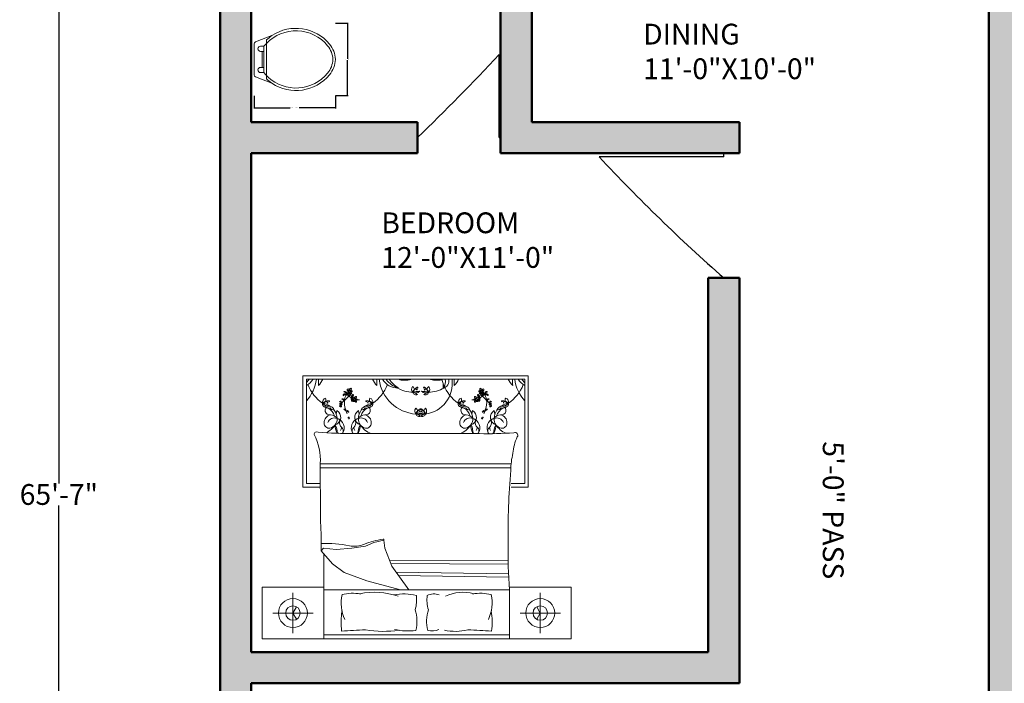
# Model space of a CAD drawing. Units: inches. Extents: x -17 to 536, y -817 to 53.
# Tile 4 of 9: x -17 to 268, y -436 to -245. Entities that reach past the tile are written whole.
import ezdxf

# ---------------------------------------------------------------- set-up
doc = ezdxf.new("R2010")
doc.units = ezdxf.units.IN
doc.header["$MEASUREMENT"] = 0
for name, color, linetype, lineweight in [('A-ANNO-DIMS', 2, 'Continuous', 18), ('A-AREA-IDEN', 7, 'Continuous', 18), ('A-DOOR', 4, 'Continuous', 25), ('A-FLOR-FIXT', 9, 'Continuous', 18), ('A-FURN', 8, 'Continuous', 13), ('A-WALL', 7, 'Continuous', 50), ('A-WALL-PATT', 22, 'Continuous', 13)]:
    doc.layers.add(name, color=color, linetype=linetype, lineweight=lineweight)
doc.styles.get("Standard").update_dxf_attribs({"font": 'arial.ttf'})
doc.dimstyles.get("Standard").update_dxf_attribs({"dimtxt": 0.18, "dimasz": 0.18, "dimexe": 0.18, "dimexo": 0.0625, "dimgap": 0.09, "dimtad": 0, "dimtih": 1, "dimtoh": 1, "dimdec": 0, "dimzin": 0, "dimdsep": 46, "dimlunit": 3, "dimtxsty": 'Standard', "dimcen": 0.09, "dimadec": 0, "dimazin": 0, "dimtfac": 1, "dimtdec": 0, "dimtofl": 0, "dimtmove": 0, "dimatfit": 3, "dimfxl": 1, "dimtolj": 1, "dimtzin": 0, "dimarcsym": 0})

# ---------------------------------------------------------------- blocks, each defined once
blk = doc.blocks.new('*D2')
at = {"layer": 'A-ANNO-DIMS', "color": 0, "lineweight": -2, "transparency": 16777216}
for p, q in [((41.3, 11.55), (-5.38, 11.55)), ((-5.2, 11.37), (-5.2, -378.8)), ((-5.2, -775.27), (-5.2, -385.1)), ((41.3, -775.45), (-5.38, -775.45))]:
    blk.add_line(p, q, dxfattribs=at)
at = {"layer": 'A-ANNO-DIMS', "color": 0, "transparency": 16777216}
for points in [[(-5.23, 11.37), (-5.17, 11.37), (-5.2, 11.55)], [(-5.23, -775.27), (-5.17, -775.27), (-5.2, -775.45)]]:
    blk.add_solid(points, dxfattribs=at)
at = {"layer": 'Defpoints', "color": 0, "transparency": 16777216}
for p in [(41.37, 11.55), (-5.2, -775.45), (41.37, -775.45)]:
    blk.add_point(p, dxfattribs=at)
at = {"layer": 'A-ANNO-DIMS', "color": 0, "transparency": 16777216, "insert": (-5.2, -381.95), "char_height": 6, "attachment_point": 5}
blk.add_mtext('\\A1;65\'-7"', dxfattribs=at)
blk = doc.blocks.new('BED-WITH-NIGHTSTANDS-STANDARD')
for p, q in [((11.79, 75.95), (11.79, 43.78)), ((76.89, 75.95), (11.79, 75.95)), ((12.82, 74.91), (75.86, 74.91)), ((12.82, 44.81), (12.82, 74.91)), ((75.86, 74.91), (75.86, 44.81)), ((76.89, 43.78), (76.89, 75.95)), ((21.62, 65.86), (21.42, 64.85)), ((27.86, 65.86), (28.06, 64.85)), ((60.82, 65.86), (60.62, 64.85)), ((67.06, 65.86), (67.25, 64.85)), ((62.78, 59.23), (26.52, 59.23)), ((71.93, 50.46), (16.83, 50.46)), ((71.85, 49.35), (16.83, 49.35)), ((11.79, 43.78), (16.84, 43.78)), ((16.84, 44.81), (12.82, 44.81)), ((75.86, 44.81), (71.92, 44.81)), ((71.94, 43.78), (76.89, 43.78)), ((35.15, 28.52), (32.25, 27.79)), ((35.51, 26.17), (35.15, 28.52)), ((17.78, 26.17), (17.06, 25.44)), ((21.4, 25.8), (17.78, 26.17)), ((25.92, 26.17), (21.4, 25.8)), ((29.9, 26.71), (25.92, 26.17)), ((32.25, 27.79), (29.9, 26.71)), ((37.5, 20.92), (35.51, 26.17)), ((17.06, 25.44), (20.32, 21.65)), ((17.86, 0), (17.86, 24.51)), ((20.32, 21.65), (23.75, 19.12)), ((71.13, 22.47), (36.86, 22.61)), ((71.12, 21.55), (37.21, 21.69)), ((42.39, 14.11), (37.5, 20.92)), ((23.75, 19.12), (30.26, 16.77)), ((71.17, 18.74), (38.74, 19.2)), ((71.2, 17.82), (39.41, 18.27)), ((30.26, 16.77), (40, 14.11)), ((8.93, 13.28), (8.93, 1.61)), ((17.86, 14.11), (71.44, 14.11)), ((80.37, 13.28), (80.37, 1.61)), ((14.76, 7.44), (3.1, 7.44)), ((74.54, 7.44), (86.21, 7.44)), ((0, 0), (89.3, 0)), ((71.44, 1.15), (17.86, 1.15))]:
    blk.add_line(p, q)
for points in [[(16.87, 33.62, -0.001242), (16.83, 50.56, 0.127202), (15.04, 59.01)], [(71.82, 48.64, -0.056112), (72.47, 53.56, -0.095341), (73.73, 58.29)], [(22.99, 2.23, -0.074897), (23.1, 8.06, 0.472817)], [(44.23, 8.39, -0.14099), (44.41, 2.43, -0.235245)], [(48.05, 8.39, 0.14099), (47.87, 2.43, 0.235245)], [(66.31, 2.23, 0.074897), (66.2, 8.06, -0.472817)]]:
    blk.add_lwpolyline(points, format="xyb")
for points in [[(17.86, 14.88), (0, 14.88), (0, 0)], [(71.44, 0), (71.44, 14.88), (89.3, 14.88), (89.3, 0)], [(8.93, 7.44), (9.97, 9.25)], [(80.37, 7.44), (79.33, 9.25)], [(8.93, 7.44), (9.97, 5.64)], [(80.37, 7.44), (79.33, 5.64)]]:
    blk.add_lwpolyline(points)
for centre, radius in [((25.29, 71.49), 0.227), ((63.39, 71.49), 0.227), ((26.78, 69.09), 0.227), ((61.9, 69.09), 0.227), ((8.93, 7.44), 4.17), ((80.37, 7.44), 4.17), ((8.93, 7.44), 2.08), ((80.37, 7.44), 2.08)]:
    blk.add_circle(centre, radius)
for centre, radius, start, end in [((7.95, 79.1), 7.08, 313.5186, 323.6964), ((9.99, 78.04), 5.68, 299.8884, 326.5383), ((4.14, 76.48), 11.66, 318.1144, 352.255), ((13.17, 76.73), 4.74, 311.0454, 337.4453), ((0.19, 74.18), 16.13, 356.3481, 2.5919), ((36.31, 76.73), 4.74, 202.5547, 228.9546), ((49.3, 74.18), 16.13, 177.4081, 183.6519), ((45.35, 76.48), 11.66, 187.745, 265.5377), ((39.5, 78.04), 5.68, 213.4617, 268.728), ((41.54, 79.1), 7.08, 216.3036, 252.1496), ((45.26, 81.09), 10.53, 215.947, 235.9877), ((41.19, 81.04), 6.41, 252.9798, 286.4569), ((43.73, 84.35), 9.48, 264.3643, 265.6213), ((48.73, 90.84), 16.94, 250.0972, 250.2783), ((45.93, 73.79), 9.03, 278.1803, 7.1364), ((50.46, 81.04), 6.41, 253.5431, 287.0202), ((47.92, 84.35), 9.48, 274.3787, 275.6357), ((42.93, 90.84), 16.94, 289.7217, 289.9028), ((47.1, 72.96), 5.22, 353.3805, 21.883), ((51.89, 74.42), 2.09, 280.9261, 13.6102), ((50.32, 74.13), 2.65, 318.0951, 17.1391), ((39.38, 74.18), 16.13, 356.3481, 2.5919), ((52.37, 76.73), 4.74, 311.0454, 337.4453), ((75.51, 76.73), 4.74, 202.5547, 228.9546), ((88.49, 74.18), 16.13, 177.4081, 183.6519), ((84.54, 76.48), 11.66, 187.745, 221.8856), ((78.69, 78.04), 5.68, 213.4617, 240.1116), ((80.73, 79.1), 7.08, 216.3036, 226.4814), ((24.09, 77.63), 11.66, 201.4092, 235.6135), ((23.83, 71.16), 0.254, 55.6077, 145.6462), ((23.65, 70.61), 0.687, 21.7087, 93.0299), ((20.03, 65.71), 6.64, 53.6254, 57.3216), ((23.86, 70.79), 0.592, 342.8042, 79.6943), ((24.82, 71.92), 0.225, 134.3732, 211.9501), ((25.23, 72.18), 0.717, 211.9501, 255.2442), ((24.83, 71.66), 0.449, 8.5614, 112.5914), ((25.04, 71.17), 0.31, 88.5719, 233.8954), ((25.01, 71.09), 0.223, 228.2946, 6.2474), ((24.96, 71.68), 0.151, 352.868, 97.094), ((24.8, 71.35), 0.313, 298.8493, 359.9355), ((24.87, 71.09), 0.358, 4.2123, 48.1587), ((25.6, 71.91), 0.375, 100.9597, 208.7804), ((25.61, 71.14), 0.379, 183.635, 258.4363), ((25.56, 71.27), 0.217, 178.1325, 268.8919), ((26.01, 71.41), 0.69, 132.3896, 156.5724), ((25.71, 71.32), 0.372, 42.3208, 130.2111), ((25.79, 71.71), 0.47, 226.3462, 279.6513), ((25.29, 72.11), 0.529, 291.6382, 4.947), ((25.3, 70.84), 0.547, 7.4968, 71.2737), ((25.7, 72.2), 0.745, 254.2829, 276.9148), ((25.64, 72.14), 0.174, 4.947, 127.5263), ((25.84, 71.44), 0.196, 279.6513, 42.3208), ((25.39, 77.63), 11.66, 304.3865, 338.5908), ((44.45, 82.73), 11.66, 242.5854, 265.5377), ((44.5, 71.97), 1.29, 140.8855, 222.2127), ((43.03, 71.93), 0.974, 301.6373, 61.4609), ((44.5, 71.14), 0.954, 76.148, 182.2415), ((46.34, 70.15), 2.95, 121.989, 161.0841), ((45.99, 63.32), 8.16, 92.7418, 107.407), ((44.3, 72.78), 1.84, 245.6899, 314.4589), ((43.49, 69.11), 1.99, 44.6273, 88.5415), ((44.47, 71.37), 0.967, 196.1963, 296.9726), ((44.7, 71.94), 0.126, 140.0755, 76.148), ((44.85, 72.52), 0.145, 288.4408, 121.989), ((44.87, 72.45), 0.0704, 171.9833, 288.4408), ((45.67, 63.32), 8.16, 72.593, 87.2582), ((47.35, 72.78), 1.84, 225.5411, 294.3101), ((46.81, 72.52), 0.145, 58.011, 251.5592), ((48.16, 69.11), 1.99, 91.4585, 135.3727), ((47.18, 71.37), 0.967, 243.0274, 343.8037), ((46.78, 72.45), 0.0704, 251.5592, 8.0167), ((46.95, 71.89), 0.076, 103.9791, 39.8091), ((45.32, 70.15), 2.95, 18.9159, 58.011), ((47.16, 71.14), 0.954, 357.7585, 103.852), ((48.62, 71.93), 0.974, 118.5391, 238.3627), ((47.15, 71.97), 1.29, 317.7873, 39.1145), ((47.2, 82.73), 11.66, 274.4623, 297.4146), ((63.28, 77.63), 11.66, 201.4092, 235.6135), ((62.84, 71.44), 0.196, 137.6792, 260.3487), ((62.97, 71.32), 0.372, 49.7889, 137.6792), ((62.89, 71.71), 0.47, 260.3487, 313.6538), ((63.38, 70.84), 0.547, 108.7263, 172.5032), ((63.39, 72.11), 0.529, 175.053, 248.3618), ((63.04, 72.14), 0.174, 52.4737, 175.053), ((62.98, 72.2), 0.745, 263.0852, 285.7171), ((63.12, 71.27), 0.217, 271.1081, 1.8675), ((62.67, 71.41), 0.69, 23.4276, 47.6104), ((63.08, 71.91), 0.375, 331.2196, 79.0403), ((63.07, 71.14), 0.379, 281.5637, 356.365), ((63.85, 71.66), 0.449, 67.4086, 171.4386), ((63.81, 71.09), 0.358, 131.8413, 175.7877), ((63.67, 71.09), 0.223, 173.7526, 311.7054), ((63.72, 71.68), 0.151, 82.906, 187.132), ((63.88, 71.35), 0.313, 180.0645, 241.1507), ((63.45, 72.18), 0.717, 284.7558, 328.0499), ((63.64, 71.17), 0.31, 306.1046, 91.4281), ((63.86, 71.92), 0.225, 328.0499, 45.6268), ((64.81, 70.79), 0.592, 100.3057, 197.1958), ((65.03, 70.61), 0.687, 86.9701, 158.2913), ((64.85, 71.16), 0.254, 34.3538, 124.3923), ((68.65, 65.71), 6.64, 122.6784, 126.3746), ((64.59, 77.63), 11.66, 304.3865, 338.5908), ((18.77, 68.29), 1.29, 110.9613, 192.2885), ((17.48, 68.98), 0.974, 271.7131, 31.5367), ((19.45, 65.79), 2.95, 92.0648, 131.1598), ((18.35, 67.57), 0.954, 46.2238, 152.3173), ((18.92, 68.17), 0.126, 110.2817, 46.2238), ((19.33, 68.52), 0.0704, 142.0591, 258.5166), ((19.35, 68.59), 0.145, 258.5166, 92.0648), ((22.68, 68.16), 0.375, 100.9597, 142.2379), ((22.36, 68.36), 0.529, 291.6382, 4.947), ((22.72, 68.39), 0.174, 4.947, 127.5263), ((17.62, 74.63), 8.48, 307.9541, 316.8459), ((23.13, 66.79), 2.52, 82.8698, 91.6736), ((23.48, 69.5), 0.469, 205.5379, 258.6744), ((22.81, 67.91), 1.41, 59.344, 79.7412), ((23.64, 70.33), 0.254, 123.0979, 213.1364), ((22.5, 67.92), 1.43, 43.6929, 51.7899), ((24.07, 69.96), 0.687, 92.3172, 160.5201), ((27.22, 64.73), 6.64, 121.1156, 124.8118), ((23.38, 68.86), 0.429, 355.7131, 81.6568), ((24, 70.22), 0.592, 82.6008, 147.1845), ((23.14, 68.48), 0.748, 27.3659, 59.344), ((23.71, 68.98), 0.182, 202.5583, 304.2343), ((23.92, 70.2), 0.263, 45.7354, 121.1156), ((31.19, 68.33), 7.4, 176.1723, 196.4158), ((27.5, 68.52), 3.71, 150.7959, 175.244), ((32.84, 60.63), 12.2, 127.8256, 137.7588), ((23.81, 70.85), 0.263, 338.2452, 53.6254), ((24.24, 70.68), 0.198, 158.2452, 340.6395), ((24.24, 70.53), 0.198, 225.7354, 48.1297), ((27.97, 72.33), 3.96, 201.7087, 206.2181), ((24.82, 69.63), 1.04, 40.9365, 112.7695), ((24.48, 69.98), 0.61, 49.3812, 95.5456), ((27.5, 68.52), 3.71, 137.5083, 145.9967), ((24.92, 70.22), 0.63, 61.1838, 141.6792), ((27.89, 73.45), 4.45, 220.182, 239.456), ((25.35, 71), 0.733, 229.3812, 289.9959), ((24.88, 70.1), 0.753, 15.6484, 62.2957), ((25.68, 70.87), 0.176, 215.0752, 14.7644), ((25.31, 70.6), 1.04, 287.889, 359.722), ((25.28, 70.11), 0.61, 305.1128, 351.2773), ((25.59, 68.99), 0.63, 3.8774, 87.1501), ((25.15, 69.23), 0.61, 352.0748, 38.2393), ((25.04, 68.75), 1.04, 343.6301, 55.4631), ((26.48, 69.05), 0.733, 172.0748, 232.6895), ((25.77, 70.21), 0.63, 271.4625, 339.4747), ((26.61, 69.9), 0.733, 110.6625, 171.2773), ((25.47, 68.96), 0.753, 318.342, 4.9894), ((26.3, 69.52), 0.225, 134.3732, 211.9501), ((27.89, 73.45), 4.45, 246.1523, 246.9499), ((26.72, 69.78), 0.717, 211.9501, 255.2442), ((26.32, 69.27), 0.449, 8.5614, 112.5914), ((26.53, 68.78), 0.31, 88.5719, 233.8954), ((25.66, 70.27), 0.753, 338.3627, 25.0101), ((26.5, 68.69), 0.223, 228.2946, 6.2474), ((26.44, 69.28), 0.151, 352.868, 97.094), ((26.29, 68.96), 0.313, 298.8493, 359.9355), ((26.36, 68.69), 0.358, 4.2123, 48.1587), ((27.09, 69.51), 0.375, 100.9597, 208.7804), ((27.1, 68.74), 0.379, 183.635, 258.4363), ((27.05, 68.88), 0.217, 178.1325, 268.8919), ((27.5, 69.01), 0.69, 132.3896, 156.5724), ((27.19, 68.93), 0.372, 42.3208, 130.2111), ((27.28, 69.31), 0.47, 226.3462, 279.6513), ((26.77, 69.71), 0.529, 291.6382, 4.947), ((26.79, 68.44), 0.547, 7.4968, 71.2737), ((27.19, 69.8), 0.745, 254.2829, 276.9148), ((27.13, 69.74), 0.174, 4.947, 127.5263), ((27.16, 68.47), 0.176, 215.0752, 14.7644), ((27.32, 69.04), 0.196, 279.6513, 42.3208), ((27.89, 73.45), 4.45, 265.2415, 272.8929), ((30.14, 68.59), 0.145, 87.9352, 281.4834), ((30.04, 65.79), 2.95, 48.8402, 87.9352), ((30.16, 68.52), 0.0704, 281.4834, 37.9409), ((31.14, 67.57), 0.954, 27.6827, 133.7762), ((32.01, 68.98), 0.974, 148.4633, 268.2869), ((30.72, 68.29), 1.29, 347.7115, 69.0387), ((57.96, 68.29), 1.29, 110.9613, 192.2885), ((56.67, 68.98), 0.974, 271.7131, 31.5367), ((58.64, 65.79), 2.95, 92.0648, 131.1598), ((57.54, 67.57), 0.954, 46.2238, 152.3173), ((58.12, 68.17), 0.126, 110.2817, 46.2238), ((58.52, 68.52), 0.0704, 142.0591, 258.5166), ((58.54, 68.59), 0.145, 258.5166, 92.0648), ((60.79, 73.45), 4.45, 267.1071, 274.7585), ((61.36, 69.04), 0.196, 137.6792, 260.3487), ((61.49, 68.93), 0.372, 49.7889, 137.6792), ((61.4, 69.31), 0.47, 260.3487, 313.6538), ((61.52, 68.47), 0.176, 165.2356, 324.9248), ((61.89, 68.44), 0.547, 108.7263, 172.5032), ((61.55, 69.74), 0.174, 52.4737, 175.053), ((61.91, 69.71), 0.529, 175.053, 248.3618), ((61.49, 69.8), 0.745, 263.0852, 285.7171), ((61.63, 68.88), 0.217, 271.1081, 1.8675), ((61.18, 69.01), 0.69, 23.4276, 47.6104), ((61.59, 69.51), 0.375, 331.2196, 79.0403), ((61.58, 68.74), 0.379, 281.5637, 356.365), ((62.36, 69.27), 0.449, 67.4086, 171.4386), ((62.32, 68.69), 0.358, 131.8413, 175.7877), ((62.18, 68.69), 0.223, 173.7526, 311.7054), ((62.23, 69.28), 0.151, 82.906, 187.132), ((62.39, 68.96), 0.313, 180.0645, 241.1507), ((61.96, 69.78), 0.717, 284.7558, 328.0499), ((62.15, 68.78), 0.31, 306.1046, 91.4281), ((63.02, 70.27), 0.753, 154.9899, 201.6373), ((62.91, 70.21), 0.63, 200.5253, 268.5375), ((63.37, 70.6), 1.04, 180.278, 252.111), ((62.07, 69.9), 0.733, 8.7227, 69.3375), ((63.21, 68.96), 0.753, 175.0106, 221.658), ((63.08, 68.99), 0.63, 92.8499, 176.1226), ((62.38, 69.52), 0.225, 328.0499, 45.6268), ((60.79, 73.45), 4.45, 293.0501, 293.8477), ((63.64, 68.75), 1.04, 124.5369, 196.3699), ((62.2, 69.05), 0.733, 307.3105, 7.9252), ((63.4, 70.11), 0.61, 188.7227, 234.8872), ((63, 70.87), 0.176, 165.2356, 324.9248), ((63.53, 69.23), 0.61, 141.7607, 187.9252), ((60.79, 73.45), 4.45, 300.544, 319.818), ((63.8, 70.1), 0.753, 117.7043, 164.3516), ((63.86, 69.63), 1.04, 67.2305, 139.0635), ((63.33, 71), 0.733, 250.0041, 310.6188), ((55.84, 60.63), 12.2, 42.2412, 52.1744), ((63.75, 70.22), 0.63, 38.3208, 118.8162), ((64.2, 69.98), 0.61, 84.4544, 130.6188), ((61.17, 68.52), 3.71, 34.0033, 42.4917), ((64.44, 70.53), 0.198, 131.8703, 314.2646), ((64.44, 70.68), 0.198, 199.3605, 21.7548), ((60.71, 72.33), 3.96, 333.7819, 338.2913), ((61.17, 68.52), 3.71, 4.756, 29.2041), ((64.76, 70.2), 0.263, 58.8844, 134.2646), ((57.49, 68.33), 7.4, 343.5842, 3.8277), ((64.86, 70.85), 0.263, 126.3746, 201.7548), ((64.68, 70.22), 0.592, 32.8155, 97.3992), ((64.6, 69.96), 0.687, 19.4799, 87.6828), ((65.3, 68.86), 0.429, 98.3432, 184.2869), ((65.53, 68.48), 0.748, 120.656, 152.6341), ((64.97, 68.98), 0.182, 235.7657, 337.4417), ((71.06, 74.63), 8.48, 223.1541, 232.0459), ((61.46, 64.73), 6.64, 55.1882, 58.8844), ((66.18, 67.92), 1.43, 128.2101, 136.3071), ((65.87, 67.91), 1.41, 100.2588, 120.656), ((65.04, 70.33), 0.254, 326.8636, 56.9021), ((65.55, 66.79), 2.52, 88.3264, 97.1302), ((65.2, 69.5), 0.469, 281.3256, 334.4621), ((65.96, 68.39), 0.174, 52.4737, 175.053), ((66.31, 68.36), 0.529, 175.053, 248.3618), ((66, 68.16), 0.375, 37.7621, 79.0403), ((69.33, 68.59), 0.145, 87.9352, 281.4834), ((69.23, 65.79), 2.95, 48.8402, 87.9352), ((69.35, 68.52), 0.0704, 281.4834, 37.9409), ((70.33, 67.57), 0.954, 27.6827, 133.7762), ((71.2, 68.98), 0.974, 148.4633, 268.2869), ((69.91, 68.29), 1.29, 347.7115, 69.0387), ((18.44, 67.78), 0.967, 166.272, 267.0484), ((15.74, 60.05), 8.16, 62.8176, 77.4827), ((19, 69.09), 1.84, 215.7657, 284.5347), ((16.47, 66.31), 1.99, 14.7031, 58.6173), ((19.58, 65.93), 1.34, 109.1312, 279.736), ((19.3, 67.38), 0.821, 216.7319, 296.0245), ((16.92, 62.98), 4.22, 18.2955, 58.7386), ((19.26, 65.53), 1.67, 15.6955, 94.031), ((21.06, 67.75), 1.78, 218.4175, 263.8338), ((16.88, 63.32), 4.79, 3.4924, 33.7117), ((20.52, 63.93), 2.22, 286.8663, 60.0915), ((22.37, 67.74), 0.227, 273.2768, 86.7232), ((22.69, 67.39), 0.379, 217.3642, 258.4363), ((22.64, 67.53), 0.217, 178.1325, 268.8919), ((23.09, 67.66), 0.69, 132.3896, 156.5724), ((22.78, 67.57), 0.372, 42.3208, 130.2111), ((22.87, 67.96), 0.47, 226.3462, 279.6513), ((22.38, 67.09), 0.547, 7.4968, 71.2737), ((22.78, 68.45), 0.745, 254.2829, 276.9148), ((22.75, 67.12), 0.176, 215.0752, 14.7644), ((22.91, 67.69), 0.196, 279.6513, 42.3208), ((23.66, 63.78), 2.52, 82.8698, 91.6736), ((24.01, 66.5), 0.469, 205.5379, 258.6744), ((23.34, 64.91), 1.41, 59.344, 79.7412), ((23.03, 64.91), 1.43, 43.6929, 51.7899), ((23.91, 65.86), 0.429, 355.7131, 81.6568), ((23.68, 65.48), 0.748, 27.3659, 59.344), ((24.24, 65.97), 0.182, 202.5583, 304.2343), ((31.19, 68.33), 7.4, 200.1059, 206.9968), ((24.57, 65.46), 0.429, 36.5232, 122.4668), ((24.35, 65.08), 0.748, 58.836, 90.8141), ((24.52, 65.8), 0.182, 173.9457, 275.6216), ((24.16, 64.24), 1.43, 66.3901, 74.4871), ((25.09, 65.85), 0.469, 219.5056, 272.6421), ((24.01, 64.51), 1.41, 38.4388, 58.836), ((22.86, 64.26), 2.52, 26.5064, 35.3102), ((28.97, 63.93), 2.22, 119.9085, 253.1337), ((32.6, 63.32), 4.79, 146.2883, 176.5076), ((32.56, 62.98), 4.22, 121.2614, 161.7045), ((30.23, 65.53), 1.67, 85.969, 164.3045), ((28.42, 67.75), 1.78, 276.1662, 321.5825), ((29.91, 65.93), 1.34, 260.264, 70.8688), ((30.18, 67.38), 0.821, 243.9755, 323.2681), ((30.48, 69.09), 1.84, 255.4653, 324.2343), ((33.75, 60.05), 8.16, 102.5173, 117.1824), ((30.58, 68.12), 0.076, 133.7729, 69.7333), ((31.04, 67.78), 0.967, 272.9516, 13.728), ((33.02, 66.31), 1.99, 121.3827, 165.2969), ((45.4, 65.72), 1.29, 140.8855, 222.2127), ((43.93, 65.68), 0.974, 301.6373, 61.4609), ((47.23, 63.9), 2.95, 121.989, 161.0841), ((45.39, 64.89), 0.954, 76.148, 182.2415), ((45.59, 65.7), 0.126, 140.0755, 76.148), ((45.74, 66.28), 0.145, 288.4408, 121.989), ((45.77, 66.21), 0.0704, 171.9833, 288.4408), ((45.91, 66.28), 0.145, 58.011, 251.5592), ((45.89, 66.21), 0.0704, 251.5592, 8.0167), ((46.05, 65.65), 0.076, 103.9791, 39.8091), ((44.43, 63.9), 2.95, 18.9159, 58.011), ((46.26, 64.89), 0.954, 357.7585, 103.852), ((47.73, 65.68), 0.974, 118.5391, 238.3627), ((46.26, 65.72), 1.29, 317.7873, 39.1145), ((57.64, 67.78), 0.967, 166.272, 267.0484), ((55.66, 66.31), 1.99, 14.7031, 58.6173), ((58.19, 69.09), 1.84, 215.7657, 284.5347), ((54.93, 60.05), 8.16, 62.8176, 77.4827), ((58.77, 65.93), 1.34, 109.1312, 279.736), ((58.5, 67.38), 0.821, 216.7319, 296.0245), ((56.12, 62.98), 4.22, 18.2955, 58.7386), ((58.45, 65.53), 1.67, 15.6955, 94.031), ((60.25, 67.75), 1.78, 218.4175, 263.8338), ((56.08, 63.32), 4.79, 3.4924, 33.7117), ((59.71, 63.93), 2.22, 286.8663, 60.0915), ((64.67, 64.51), 1.41, 121.164, 141.5612), ((65.82, 64.26), 2.52, 144.6898, 153.4936), ((63.59, 65.85), 0.469, 267.3579, 320.4944), ((64.11, 65.46), 0.429, 57.5332, 143.4768), ((64.33, 65.08), 0.748, 89.1859, 121.164), ((64.52, 64.24), 1.43, 105.5129, 113.6099), ((57.49, 68.33), 7.4, 333.0032, 339.8941), ((64.16, 65.8), 0.182, 264.3784, 6.0543), ((64.77, 65.86), 0.429, 98.3432, 184.2869), ((65, 65.48), 0.748, 120.656, 152.6341), ((64.44, 65.97), 0.182, 235.7657, 337.4417), ((65.65, 64.91), 1.43, 128.2101, 136.3071), ((65.34, 64.91), 1.41, 100.2588, 120.656), ((65.02, 63.78), 2.52, 88.3264, 97.1302), ((64.67, 66.5), 0.469, 281.3256, 334.4621), ((65.76, 67.69), 0.196, 137.6792, 260.3487), ((65.89, 67.57), 0.372, 49.7889, 137.6792), ((65.81, 67.96), 0.47, 260.3487, 313.6538), ((66.3, 67.09), 0.547, 108.7263, 172.5032), ((65.92, 67.12), 0.176, 165.2356, 324.9248), ((65.9, 68.45), 0.745, 263.0852, 285.7171), ((68.16, 63.93), 2.22, 119.9085, 253.1337), ((66.04, 67.53), 0.217, 271.1081, 1.8675), ((65.59, 67.66), 0.69, 23.4276, 47.6104), ((65.99, 67.39), 0.379, 281.5637, 322.6358), ((66.31, 67.74), 0.227, 93.2768, 266.7232), ((71.8, 63.32), 4.79, 146.2883, 176.5076), ((71.76, 62.98), 4.22, 121.2614, 161.7045), ((69.42, 65.53), 1.67, 85.969, 164.3045), ((67.62, 67.75), 1.78, 276.1662, 321.5825), ((69.1, 65.93), 1.34, 260.264, 70.8688), ((69.38, 67.38), 0.821, 243.9755, 323.2681), ((72.94, 60.05), 8.16, 102.5173, 117.1824), ((69.68, 69.09), 1.84, 255.4653, 324.2343), ((69.77, 68.12), 0.076, 133.7729, 69.7333), ((72.21, 66.31), 1.99, 121.3827, 165.2969), ((70.23, 67.78), 0.967, 272.9516, 13.728), ((20.07, 62.49), 2.13, 97.1143, 185.0551), ((20.91, 61.68), 2.07, 68.5779, 158.4181), ((18.99, 63.39), 2.69, 283.079, 4.7067), ((19.7, 62.02), 2.59, 35.9599, 87.6409), ((24.57, 61.5), 3.44, 143.6555, 147.2989), ((21.92, 63), 0.554, 344.8529, 102.6959), ((20.86, 60.85), 2.85, 330.8249, 70.7178), ((24.22, 62.38), 1.83, 164.8529, 228.4347), ((25, 63.84), 0.172, 79.5616, 257.2949), ((24.98, 63.73), 0.28, 259.5864, 79.5616), ((28.63, 60.85), 2.85, 109.2822, 209.1751), ((25.26, 62.38), 1.83, 311.5653, 15.1471), ((27.56, 63), 0.554, 77.3041, 195.1471), ((29.79, 62.02), 2.59, 92.3591, 144.0401), ((24.91, 61.5), 3.44, 32.7011, 36.3445), ((30.5, 63.39), 2.69, 175.2933, 256.921), ((28.58, 61.68), 2.07, 21.5819, 111.4221), ((29.42, 62.49), 2.13, 354.9449, 82.8857), ((45.2, 66.54), 1.84, 245.6899, 314.4589), ((46.88, 57.07), 8.16, 92.7418, 107.407), ((45.37, 65.13), 0.967, 196.1963, 296.9726), ((44.39, 62.86), 1.99, 44.6273, 88.5415), ((46.46, 66.54), 1.84, 225.5411, 294.3101), ((44.78, 57.07), 8.16, 72.593, 87.2582), ((46.29, 65.13), 0.967, 243.0274, 343.8037), ((47.27, 62.86), 1.99, 91.4585, 135.3727), ((59.26, 62.49), 2.13, 97.1143, 185.0551), ((60.1, 61.68), 2.07, 68.5779, 158.4181), ((58.18, 63.39), 2.69, 283.079, 4.7067), ((58.89, 62.02), 2.59, 35.9599, 87.6409), ((63.77, 61.5), 3.44, 143.6555, 147.2989), ((61.11, 63), 0.554, 344.8529, 102.6959), ((60.05, 60.85), 2.85, 330.8249, 70.7178), ((63.42, 62.38), 1.83, 164.8529, 228.4347), ((63.7, 63.73), 0.28, 100.4384, 280.4136), ((63.68, 63.84), 0.172, 282.7051, 100.4384), ((67.82, 60.85), 2.85, 109.2822, 209.1751), ((64.46, 62.38), 1.83, 311.5653, 15.1471), ((66.76, 63), 0.554, 77.3041, 195.1471), ((68.98, 62.02), 2.59, 92.3591, 144.0401), ((64.11, 61.5), 3.44, 32.7011, 36.3445), ((69.69, 63.39), 2.69, 175.2933, 256.921), ((67.77, 61.68), 2.07, 21.5819, 111.4221), ((68.61, 62.49), 2.13, 354.9449, 82.8857), ((15.86, 58.95), 0.824, 62.6588, 176.02), ((19.45, 62.27), 1.51, 178.9462, 275.5144), ((15.52, 65.52), 6.76, 296.7003, 326.3329), ((24.57, 61.5), 3.44, 175.2696, 214.215), ((17.99, 59.89), 3.7, 350.8446, 31.1782), ((20.43, 61.37), 2.57, 330.0851, 352.564), ((22.12, 60.01), 1.34, 336.1646, 48.4347), ((27.36, 60.01), 1.34, 131.5653, 203.8354), ((29.06, 61.37), 2.57, 187.436, 209.9149), ((24.91, 61.5), 3.44, 325.785, 4.7304), ((31.49, 59.89), 3.7, 148.8218, 190.2867), ((33.97, 65.52), 6.76, 213.6671, 248.5059), ((30.03, 62.27), 1.51, 264.4856, 1.0538), ((58.65, 62.27), 1.51, 178.9462, 275.5144), ((54.71, 65.52), 6.76, 291.4941, 326.3329), ((63.77, 61.5), 3.44, 175.2696, 214.215), ((57.19, 59.89), 3.7, 349.7133, 31.1782), ((59.62, 61.37), 2.57, 330.0851, 352.564), ((61.32, 60.01), 1.34, 336.1646, 48.4347), ((66.56, 60.01), 1.34, 131.5653, 203.8354), ((68.25, 61.37), 2.57, 187.436, 209.9149), ((64.11, 61.5), 3.44, 325.785, 4.7304), ((70.68, 59.89), 3.7, 148.8218, 190.751), ((73.16, 65.52), 6.76, 213.6671, 246.3547), ((69.23, 62.27), 1.51, 264.4856, 1.0538), ((25.46, 152.19), 92.96, 264.3113, 270.6567), ((22.58, 60.22), 1.08, 217.675, 239.9707), ((22.58, 60.22), 1.08, 296.442, 315.5483), ((26.91, 60.22), 1.08, 224.4517, 246.771), ((26.91, 60.22), 1.08, 293.2856, 322.325), ((61.77, 60.22), 1.08, 217.675, 246.7144), ((61.77, 60.22), 1.08, 293.2856, 315.5483), ((65.51, 146.09), 86.9, 268.1965, 274.7598), ((66.1, 60.22), 1.08, 224.4517, 253.3657), ((66.1, 60.22), 1.08, 287.4186, 322.325), ((73.05, 58.74), 0.814, 326.1736, 113.4781), ((280.38, 30.86), 209.31, 175.1265, 180.8855), ((-64.82, 27.66), 81.91, 358.447, 4.1706), ((41.35, -5.23), 34.63, 100.6617, 109.8806), ((34.95, 28.59), 0.215, 340.2464, 91.1377), ((18.59, -6.18), 33.7, 78.6608, 92.5481), ((26.65, 33.99), 7.27, 258.6608, 293.7384), ((231.53, 25.03), 160.46, 179.0718, 183.9), ((34.37, 10.4), 11.51, 168.2417, 204.8684), ((26.18, 1.18), 11.97, 78.9631, 104.8961), ((32.48, -7.33), 20.76, 70.7385, 101.9603), ((40.88, -2.79), 15.75, 76.3762, 100.1383), ((33.71, 11.37), 10.94, 344.1707, 5.9871), ((58.57, 11.37), 10.94, 174.0129, 195.8293), ((49.69, 8.22), 4.73, 71.4593, 114.9817), ((57.96, 2.06), 11.37, 73.8254, 116.1239), ((63.13, 1.18), 11.97, 75.1039, 101.0369), ((54.94, 10.4), 11.51, 335.1316, 11.7583), ((72.21, -847.63), 851.28, 92.85022, 93.31479), ((35.23, 34.54), 32.39, 260.503, 277.7804), ((42.07, 18.17), 15.91, 256.04, 278.4751), ((49.09, 6.68), 4.42, 253.8974, 296.6563), ((55.71, 17.85), 15.7, 258.8159, 283.6573), ((17.09, -847.63), 851.28, 86.68521, 87.14978)]:
    blk.add_arc(centre, radius, start, end)
blk = doc.blocks.new('WC-23IN')
for p, q in [((3.55, 13.58), (3.55, 14.57)), ((3.55, 13.58), (3.55, 8.97)), ((3.55, 4.35), (3.55, 8.97)), ((3.55, 3.36), (3.55, 4.35))]:
    blk.add_line(p, q)
for points in [[(3.55, 13.58, -0.448546), (21.24, 12.93, -0.162618), (22.76, 8.97, -0.470877)], [(5.16, 15.84, -0.383919), (21.78, 13.38, -0.163732), (23.47, 8.97, -0.359733)], [(0, 8.97), (0, 13.45, -0.31031), (0.38, 14), (5.16, 15.84, -0.209071)], [(3.55, 14.57, -0.040937), (5.16, 15.84, -0.163732)], [(2.84, 12.77), (1.86, 12.77, 1), (1.86, 11.28), (2.37, 11.28)], [(2.84, 12.77, -0.022712), (3.55, 13.58, -0.162618)], [(2.84, 8.97), (2.84, 12.77, -0.476108)], [(0, 8.97), (0, 4.48, 0.31031), (0.38, 3.94), (5.16, 2.09, 0.209071)], [(2.84, 8.97), (2.84, 5.16, 0.022712)], [(4.03, 3.88, 0.431639), (21.24, 5, 0.162618), (22.76, 8.97, 0.470877)], [(5.16, 2.09, 0.383919), (21.78, 4.55, 0.163732), (23.47, 8.97, 0.359733)], [(2.84, 5.16), (1.86, 5.16, -1), (1.86, 6.66), (2.37, 6.66)], [(2.84, 5.16, 0.022712), (3.55, 4.35, 0.162618)], [(3.55, 4.35, 0.014165), (4.03, 3.88, 0.162618)], [(3.55, 3.36, 0.040937), (5.16, 2.09, 0.163732)]]:
    blk.add_lwpolyline(points, format="xyb")
for points in [[(2.37, 11.28), (2.37, 6.66)], [(2.37, 11.28), (2.84, 11.28)], [(2.37, 6.66), (2.84, 6.66)]]:
    blk.add_lwpolyline(points)
blk = doc.blocks.new('*D22')
at = {"layer": 'A-ANNO-DIMS', "color": 0, "lineweight": -2, "transparency": 16777216}
for p, q in [((51.19, -266.85), (51.19, -270.49)), ((74.66, -266.85), (74.66, -270.49)), ((51.37, -270.31), (61.64, -270.31)), ((74.48, -270.31), (64.21, -270.31))]:
    blk.add_line(p, q, dxfattribs=at)
at = {"layer": 'A-ANNO-DIMS', "color": 0, "transparency": 16777216}
for points in [[(51.37, -270.28), (51.37, -270.34), (51.19, -270.31)], [(74.48, -270.28), (74.48, -270.34), (74.66, -270.31)]]:
    blk.add_solid(points, dxfattribs=at)
at = {"layer": 'Defpoints', "color": 0, "transparency": 16777216}
for p in [(51.19, -266.79), (74.66, -266.79), (74.66, -270.31)]:
    blk.add_point(p, dxfattribs=at)
at = {"layer": 'A-ANNO-DIMS', "color": 0, "transparency": 16777216, "insert": (62.93, -270.31), "char_height": 0.18, "attachment_point": 5}
blk.add_mtext('\\A1;WC A 1\'-11 1/2" TYP.', dxfattribs=at)
blk = doc.blocks.new('*D23')
at = {"layer": 'A-ANNO-DIMS', "color": 0, "lineweight": -2, "transparency": 16777216}
for p, q in [((74.72, -245.94), (78.36, -245.94)), ((78.18, -246.12), (78.18, -256.18)), ((78.18, -266.61), (78.18, -256.55)), ((74.72, -266.79), (78.36, -266.79))]:
    blk.add_line(p, q, dxfattribs=at)
at = {"layer": 'A-ANNO-DIMS', "color": 0, "transparency": 16777216}
for points in [[(78.15, -246.12), (78.21, -246.12), (78.18, -245.94)], [(78.15, -266.61), (78.21, -266.61), (78.18, -266.79)]]:
    blk.add_solid(points, dxfattribs=at)
at = {"layer": 'Defpoints', "color": 0, "transparency": 16777216}
for p in [(74.66, -245.94), (78.18, -245.94), (74.66, -266.79)]:
    blk.add_point(p, dxfattribs=at)
at = {"layer": 'A-ANNO-DIMS', "color": 0, "transparency": 16777216, "insert": (78.18, -256.36), "char_height": 0.18, "attachment_point": 5}
blk.add_mtext('\\A1;1\'-9" TYP.', dxfattribs=at)

msp = doc.modelspace()

# ---------------------------------------------------------------- hatches: boundary and pattern name
at = {"layer": 'A-WALL-PATT'}
h = msp.add_hatch(color=256, dxfattribs=at)
h.dxf.hatch_style = 1
h.paths.add_polyline_path([(217.37, -544.45), (208.37, -544.45), (208.37, -775.45), (217.37, -775.45)], flags=17)
h.paths.add_polyline_path([(327.37, -544.45), (318.37, -544.45), (318.37, -775.45), (327.37, -775.45)], flags=17)
h.paths.add_polyline_path([(494.37, 11.55), (41.37, 11.55), (41.37, -775.45), (50.37, -775.45), (50.37, -739.45), (184.37, -739.45), (184.37, -730.45), (50.37, -730.45), (50.37, -610.45), (172.37, -610.45), (172.37, -601.45), (155.37, -601.45), (155.37, -577.45), (146.37, -577.45), (146.37, -601.45), (50.37, -601.45), (50.37, -553.45), (172.37, -553.45), (172.37, -544.45), (50.37, -544.45), (50.37, -436.45), (191.37, -436.45), (191.37, -319.45), (182.37, -319.45), (182.37, -427.45), (50.37, -427.45), (50.37, -283.45), (98.37, -283.45), (98.37, -274.45), (50.37, -274.45), (50.37, -219.45), (122.37, -219.45), (122.37, -283.45), (191.37, -283.45), (191.37, -274.45), (131.37, -274.45), (131.37, -219.45), (131.37, -150.45), (146.37, -150.45), (146.37, -141.45), (122.37, -141.45), (122.37, -210.45), (50.37, -210.45), (50.37, -150.45), (98.37, -150.45), (98.37, -141.45), (50.37, -141.45), (50.37, 2.55), (182.37, 2.55), (182.37, -150.45), (191.37, -150.45), (191.37, 2.55), (263.37, 2.55), (263.37, -141.45), (227.37, -141.45), (227.37, -150.45), (263.37, -150.45), (263.37, -553.45), (272.37, -553.45), (272.37, -150.45), (308.37, -150.45), (308.37, -141.45), (272.37, -141.45), (272.37, 2.55), (344.37, 2.55), (344.37, -150.45), (353.37, -150.45), (353.37, 2.55), (485.37, 2.55), (485.37, -141.45), (437.37, -141.45), (437.37, -150.45), (485.37, -150.45), (485.37, -210.45), (413.37, -210.45), (413.37, -141.45), (389.37, -141.45), (389.37, -150.45), (404.37, -150.45), (404.37, -219.45), (404.37, -274.45), (353.37, -274.45), (344.37, -274.45), (344.37, -283.45), (353.37, -283.45), (413.37, -283.45), (413.37, -219.45), (485.37, -219.45), (485.37, -274.45), (437.37, -274.45), (437.37, -283.45), (485.37, -283.45), (485.37, -427.45), (353.37, -427.45), (353.37, -319.45), (344.37, -319.45), (344.37, -436.45), (485.37, -436.45), (485.37, -544.45), (363.37, -544.45), (363.37, -553.45), (485.37, -553.45), (485.37, -601.45), (389.37, -601.45), (389.37, -577.45), (380.37, -577.45), (380.37, -601.45), (363.37, -601.45), (363.37, -610.45), (485.37, -610.45), (485.37, -730.45), (351.37, -730.45), (351.37, -739.45), (485.37, -739.45), (485.37, -775.45), (494.37, -775.45)])

# ---------------------------------------------------------------- linework, layer by layer
at = {"layer": 'A-DOOR'}
for p, q in [((121.97, -278.95), (121.97, -254.95)), ((121.97, -278.95), (122.37, -278.95)), ((186.87, -284.49), (186.87, -283.45)), ((186.87, -284.49), (150.87, -284.49))]:
    msp.add_line(p, q, dxfattribs=at)
for centre, radius, start, end in [((-362.2, 197.64), 662.77, 314.02027, 316.93069), ((513.73, 53.16), 495.66, 222.9393, 228.7424)]:
    msp.add_arc(centre, radius, start, end, dxfattribs=at)
at = {"layer": 'A-WALL'}
for p, q in [((41.37, 11.55), (41.37, -775.45)), ((263.37, -150.45), (263.37, -553.45)), ((50.37, -219.45), (50.37, -274.45)), ((122.37, -219.45), (122.37, -283.45)), ((131.37, -219.45), (131.37, -274.45)), ((50.37, -274.45), (98.37, -274.45)), ((98.37, -274.45), (98.37, -283.45)), ((131.37, -274.45), (191.37, -274.45)), ((191.37, -274.45), (191.37, -283.45)), ((50.37, -283.45), (98.37, -283.45)), ((50.37, -283.45), (50.37, -427.45)), ((122.37, -283.45), (191.37, -283.45)), ((182.37, -319.45), (182.37, -427.45)), ((191.37, -319.45), (182.37, -319.45)), ((191.37, -319.45), (191.37, -436.45)), ((50.37, -427.45), (182.37, -427.45)), ((50.37, -436.45), (191.37, -436.45)), ((50.37, -436.45), (50.37, -544.45))]:
    msp.add_line(p, q, dxfattribs=at)

# ---------------------------------------------------------------- block references
at = {"layer": 'A-FLOR-FIXT'}
msp.add_blockref('WC-23IN', (51.19, -265.33), dxfattribs=at)
at = {"layer": 'A-FURN'}
msp.add_blockref('BED-WITH-NIGHTSTANDS-STANDARD', (53.48, -423.61), dxfattribs=at)

# ---------------------------------------------------------------- texts
at = {"layer": 'A-AREA-IDEN', "char_height": 6, "attachment_point": 1}
for s, insert in [('DINING\\P11\'-0"X10\'-0"', (163.56, -246.07)), ('BEDROOM\\P12\'-0"X11\'-0"', (87.93, -300.53))]:
    msp.add_mtext(s, dxfattribs=dict(at, insert=insert))
at = {"layer": 'A-AREA-IDEN', "insert": (221.45, -366.6), "char_height": 6, "attachment_point": 1, "rotation": 270}
msp.add_mtext('5\'-0" PASS', dxfattribs=at)

# ---------------------------------------------------------------- dimensions: what is measured, and where the dimension line sits
at = {"layer": 'A-ANNO-DIMS'}
dim = msp.add_linear_dim(base=(-5.2, -775.45), p1=(41.37, 11.55), p2=(41.37, -775.45), angle=90, dimstyle='Standard', override={"dimtxt": 6, "dimclrd": 0, "dimclre": 0, "dimclrt": 0}, dxfattribs=at)
dim.commit()
dim.dimension.update_dxf_attribs({"geometry": '*D2', "text_midpoint": (-5.2, -381.95)})
dim = msp.add_linear_dim(base=(78.1793, -245.9388), p1=(74.6592, -266.7875), p2=(74.6592, -245.9388), angle=90, text='<> TYP.', dimstyle='Standard', override={"dimdec": 1, "dimlfac": 1, "dimrnd": 0, "dimzin": 1, "dimdsep": 46, "dimlunit": 4, "dimfrac": 2}, dxfattribs=at)
dim.commit()
dim.dimension.update_dxf_attribs({"geometry": '*D23', "text_midpoint": (78.1793, -256.3632)})
dim = msp.add_linear_dim(base=(74.66, -270.31), p1=(51.19, -266.79), p2=(74.66, -266.79), text='WC A <> TYP.', dimstyle='Standard', override={"dimdec": 1, "dimlfac": 1, "dimrnd": 0, "dimzin": 1, "dimdsep": 46, "dimlunit": 4, "dimfrac": 2}, dxfattribs=at)
dim.commit()
dim.dimension.update_dxf_attribs({"geometry": '*D22', "text_midpoint": (62.93, -270.31)})

doc.saveas('drawing.dxf')
